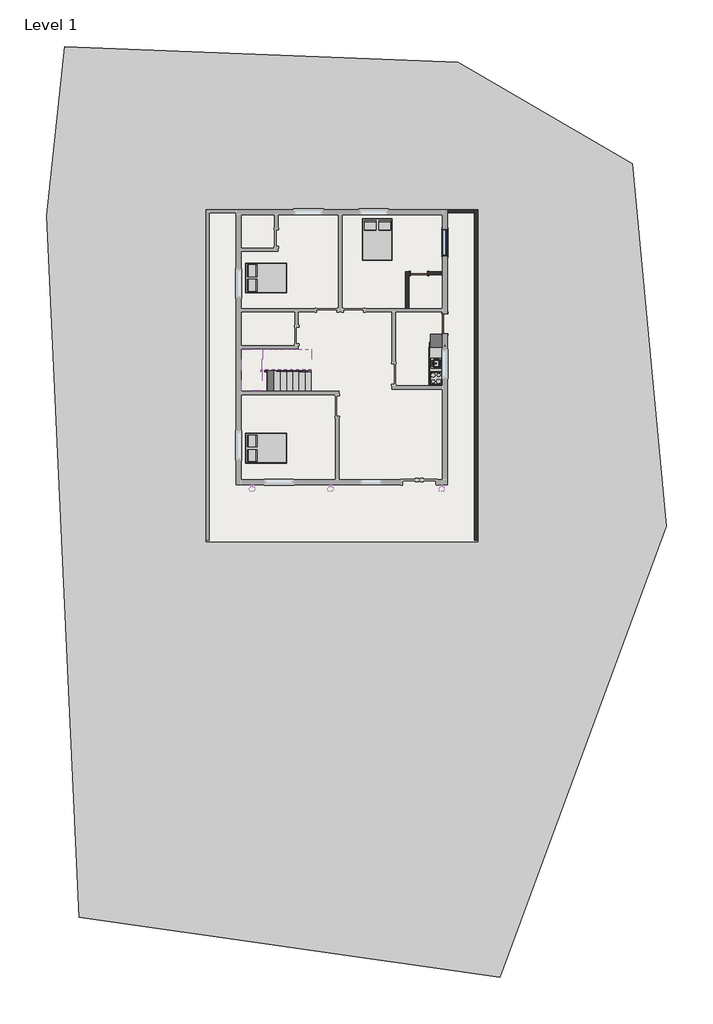
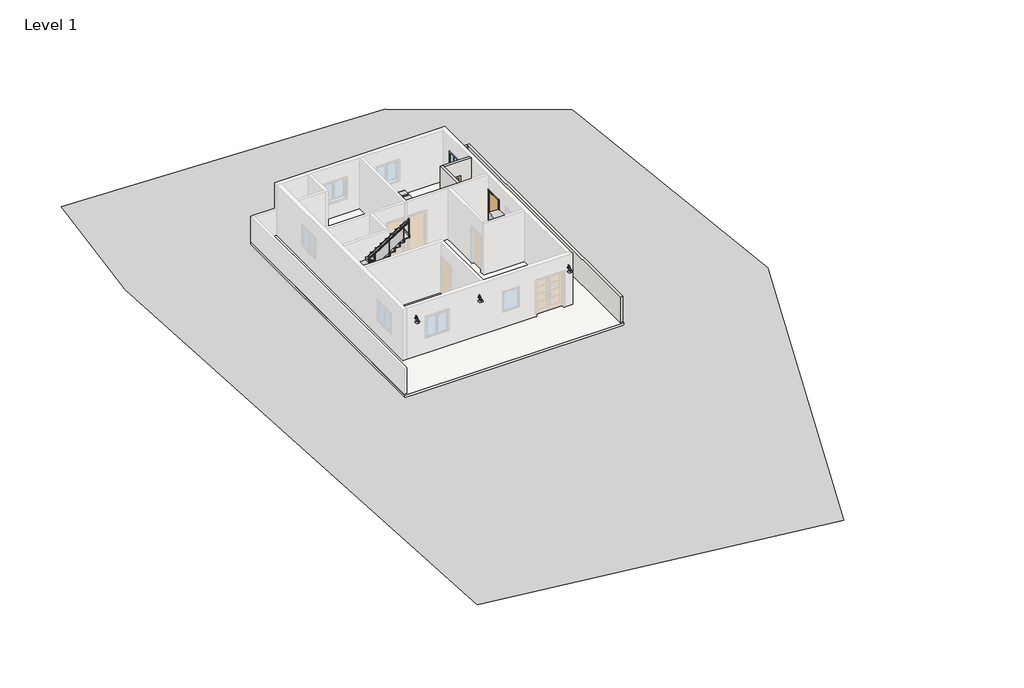
# One storey, part 2 of 2: 5 proxies, 4 furniture elements, 4 walls, 3 light fixtures, 2 doors, 2 members, 2 slabs, 2 stair flights, 3 other elements.
"""IFC4 building model written with IfcOpenShell, lengths in millimetres."""

from ifc_helpers import new_model, si_unit, frame, origin, origin_with_axes, place, context, project, spatial, polyline, outline, extrude, faceted_brep, triangles, transform, mapped, element, save
from components import proxy_a6faaae8, proxy_45b28599, kitchenette_medium_kitchenette_medium_844211aa, proxy_c523a7b7, single_flush_2_5_a9addea7, door_0ca8825f, flow_terminal_871c2e40, furniture_c8abb964, furniture_f14924cf, wall_lamp_bracket_100w_120v_38ba4611, non_monolithic_landing_7588ffe4, stair_flight_6c774f9d, stair_flight_3143a382, window_8af0dca1

model = new_model("IFC4")

# Units and contexts
model_context = context("Model", 3, world=origin())
ifc_project = project(units=[si_unit("LENGTHUNIT", "METRE", prefix="MILLI")], contexts=[model_context])

# Site, building, storey
site = spatial("IfcSite", under=ifc_project)
building = spatial("IfcBuilding", under=site)
storey = spatial("IfcBuildingStorey", under=building, Name="Level 1", Elevation=0.0)

# Proxies
placement = place(None, origin())
element("IfcBuildingElementProxy", 1, Name="Building Element Proxy", at=placement, inside=storey, context=model_context, shape_type="Tessellation", body=[
    triangles([(-15499.5818298, 15063.152655, -152.4), (2359.9797867, 14353.5017853, -152.4), (10284.4210876, 9740.7676437, -152.4), (11821.9993286, -6699.4910706, -152.4), (4274.6428596, -27186.3498779, -152.4), (-14834.2491852, -24452.2749023, -152.4), (-16327.5080383, 7375.2626129, -152.4)], [[1, 7, 2], [4, 7, 6], [4, 2, 7], [3, 2, 4], [4, 6, 5]], closed=False),
])
proxy_shape = proxy_a6faaae8(model_context)
element("IfcBuildingElementProxy", 2, Name="Cook Top-4 Unit2 : 22\" x 20\"", ObjectType="Cook Top-4 Unit2 : 22\" x 20\"", at=placement, inside=storey, context=model_context, shape_type="MappedRepresentation", body=[
    mapped(proxy_shape, transform((1354.3352982, 8.7325188, 0.0), x_axis=(0.0, 1.0000000000000002, 0.0), y_axis=(-1.0000000000000002, 0.0, 0.0), z_axis=(0.0, 0.0, 1.0))),
])
proxy_2_shape = proxy_45b28599(model_context)
element("IfcBuildingElementProxy", 3, Name="Dishwasher : 24\" x 24\" x 34\"", ObjectType="Dishwasher : 24\" x 24\" x 34\"", at=placement, inside=storey, context=model_context, shape_type="MappedRepresentation", body=[
    mapped(proxy_2_shape, transform((1646.184863, 959.9150503, 0.0), x_axis=(0.0, 1.0000000000000002, 0.0), y_axis=(-1.0000000000000002, 0.0, 0.0), z_axis=(0.0, 0.0, 1.0))),
])
kitchenette_medium_kitchenette_medium_shape = kitchenette_medium_kitchenette_medium_844211aa(model_context)
element("IfcBuildingElementProxy", 4, Name="Kitchenette - Medium : Kitchenette - Medium", ObjectType="Kitchenette - Medium : Kitchenette - Medium", at=placement, inside=storey, context=model_context, shape_type="MappedRepresentation", body=[
    mapped(kitchenette_medium_kitchenette_medium_shape, transform((1049.5352982, 332.8948139, 0.0), x_axis=(0.0, 1.0000000000000002, 0.0), y_axis=(-1.0000000000000002, 0.0, 0.0), z_axis=(0.0, 0.0, 1.0))),
])
proxy_3_shape = proxy_c523a7b7(model_context)
element("IfcBuildingElementProxy", 5, Name="Refrigerator : 24\" x 25\" LH", ObjectType="Refrigerator : 24\" x 25\" LH", at=placement, inside=storey, context=model_context, shape_type="MappedRepresentation", body=[
    mapped(proxy_3_shape, transform((1399.9842697, 1716.8825188, 0.0), x_axis=(0.0, 1.0000000000000002, 0.0), y_axis=(-1.0000000000000002, 0.0, 0.0), z_axis=(0.0, 0.0, 1.0))),
])

# Doors
single_flush_2_5_shape = single_flush_2_5_a9addea7(model_context)
element("IfcDoor", 6, ObjectType="Single-Flush : 2.5'", at=placement, inside=storey, context=model_context, shape_type="MappedRepresentation", body=[
    mapped(single_flush_2_5_shape, transform((592.3352982, 4771.2325188, 0.0), x_axis=(-1.0, 0.0, 0.0), y_axis=(0.0, -1.0, 0.0), z_axis=(0.0, 0.0, 1.0))),
])
door_shape = door_0ca8825f(model_context)
element("IfcDoor", 7, ObjectType="Single-Flush : 36\" x 84\"", at=placement, inside=storey, context=model_context, shape_type="MappedRepresentation", body=[
    mapped(door_shape, transform((1773.4352982, 2485.2325188, 0.0), x_axis=(0.0, 1.0, 0.0), y_axis=(-1.0, 0.0, 0.0), z_axis=(0.0, 0.0, 1.0))),
])

# Flow terminal
flow_terminal_shape = flow_terminal_871c2e40(model_context)
element("IfcFlowTerminal", 8, ObjectType="Sink Kitchen-Island : 18\" x 18\"", at=placement, inside=storey, context=model_context, shape_type="MappedRepresentation", body=[
    mapped(flow_terminal_shape, transform((1356.6806993, 666.1432782, -14.4), x_axis=(0.0, 1.0000000000000002, 0.0), y_axis=(-1.0000000000000002, 0.0, 0.0), z_axis=(0.0, 0.0, 1.0))),
])

# Furniture
furniture_shape = furniture_c8abb964(model_context)
element("IfcFurniture", 9, ObjectType="Bed-Box : Double 53\" x 74\"", at=placement, inside=storey, context=model_context, shape_type="MappedRepresentation", body=[
    mapped(furniture_shape, transform((-6588.99421, 4216.1800598, 0.0), x_axis=(0.0, 1.0, 0.0), y_axis=(-1.0, 0.0, 0.0), z_axis=(0.0, 0.0, 1.0))),
])
element("IfcFurniture", 10, ObjectType="Bed-Box : Double 53\" x 74\"", at=placement, inside=storey, context=model_context, shape_type="MappedRepresentation", body=[
    mapped(furniture_shape, transform((-1639.1171608, 6542.362027, 0.0), x_axis=(1.0000000000000004, 0.0, 0.0), y_axis=(0.0, 1.0000000000000004, 0.0), z_axis=(0.0, 0.0, 1.0))),
])
element("IfcFurniture", 11, ObjectType="Bed-Box : Double 53\" x 74\"", at=placement, inside=storey, context=model_context, shape_type="MappedRepresentation", body=[
    mapped(furniture_shape, transform((-6588.99421, -3504.8975153, 0.0), x_axis=(0.0, 1.0, 0.0), y_axis=(-1.0, 0.0, 0.0), z_axis=(0.0, 0.0, 1.0))),
])
furniture_2_shape = furniture_f14924cf(model_context)
element("IfcFurniture", 12, ObjectType="Counter Top w Sink Hole : 24\" Depth", at=placement, inside=storey, context=model_context, shape_type="MappedRepresentation", body=[
    mapped(furniture_2_shape, transform((1049.5352982, 866.2948139, -14.4), x_axis=(0.0, 1.0000000000000002, 0.0), y_axis=(-1.0000000000000002, 0.0, 0.0), z_axis=(0.0, 0.0, 1.0))),
])

# Light fixtures
wall_lamp_bracket_100w_120v_shape = wall_lamp_bracket_100w_120v_38ba4611(model_context)
element("IfcLightFixture", 13, ObjectType="Wall Lamp - Bracket : 100W - 120V", at=placement, inside=storey, context=model_context, shape_type="MappedRepresentation", body=[
    mapped(wall_lamp_bracket_100w_120v_shape, transform((-3461.1148241, -4715.6674812, 0.0), x_axis=(-1.0, 0.0, 0.0), y_axis=(0.0, -1.0, 0.0), z_axis=(0.0, 0.0, 1.0))),
])
element("IfcLightFixture", 14, ObjectType="Wall Lamp - Bracket : 100W - 120V", at=placement, inside=storey, context=model_context, shape_type="MappedRepresentation", body=[
    mapped(wall_lamp_bracket_100w_120v_shape, transform((-7025.9203645, -4715.6674812, 0.0), x_axis=(-1.0, 0.0, 0.0), y_axis=(0.0, -1.0, 0.0), z_axis=(0.0, 0.0, 1.0))),
])
element("IfcLightFixture", 15, ObjectType="Wall Lamp - Bracket : 100W - 120V", at=placement, inside=storey, context=model_context, shape_type="MappedRepresentation", body=[
    mapped(wall_lamp_bracket_100w_120v_shape, transform((1584.6796355, -4715.6674812, 0.0), x_axis=(-1.0, 0.0, 0.0), y_axis=(0.0, -1.0, 0.0), z_axis=(0.0, 0.0, 1.0))),
])

# Members
element("IfcMember", 16, ObjectType="Stringer - 2\" Width", at=placement, inside=storey, context=model_context, shape_type="Brep", body=[
    faceted_brep([(-4345.5091614, 301.3549437, 0.0), (-4543.6146908, 301.3549437, 0.0), (-4543.6146908, 352.1549437, 0.0), (-4345.5091614, 352.1549437, 0.0), (-6548.9591614, 301.3549437, 1371.6), (-6548.9591614, 301.3549437, 1276.1282995), (-4345.5091614, 301.3549437, 127.0), (-4624.9091614, 301.3549437, 127.0), (-4624.9091614, 301.3549437, 304.8), (-4904.3091614, 301.3549437, 304.8), (-4904.3091614, 301.3549437, 482.6), (-5183.7091614, 301.3549437, 482.6), (-5183.7091614, 301.3549437, 660.4), (-5463.1091614, 301.3549437, 660.4), (-5463.1091614, 301.3549437, 838.2), (-5742.5091614, 301.3549437, 838.2), (-5742.5091614, 301.3549437, 1016.0), (-6021.9091614, 301.3549437, 1016.0), (-6021.9091614, 301.3549437, 1193.8), (-6301.3091614, 301.3549437, 1193.8), (-6301.3091614, 301.3549437, 1371.6), (-6548.9591614, 352.1549437, 1276.1282995), (-6548.9591614, 352.1549437, 1371.6), (-6301.3091614, 352.1549437, 1118.532845), (-6021.9091614, 352.1549437, 940.732845), (-5742.5091614, 352.1549437, 762.932845), (-5463.1091614, 352.1549437, 585.132845), (-5183.7091614, 352.1549437, 407.332845), (-4904.3091614, 352.1549437, 229.532845), (-4624.9091614, 352.1549437, 51.732845), (-4345.5091614, 352.1549437, 127.0), (-4624.9091614, 352.1549437, 127.0), (-4624.9091614, 352.1549437, 304.8), (-4904.3091614, 352.1549437, 304.8), (-4904.3091614, 352.1549437, 482.6), (-5183.7091614, 352.1549437, 482.6), (-5183.7091614, 352.1549437, 660.4), (-5463.1091614, 352.1549437, 660.4), (-5463.1091614, 352.1549437, 838.2), (-5742.5091614, 352.1549437, 838.2), (-5742.5091614, 352.1549437, 1016.0), (-6021.9091614, 352.1549437, 1016.0), (-6021.9091614, 352.1549437, 1193.8), (-6301.3091614, 352.1549437, 1193.8), (-6301.3091614, 352.1549437, 1371.6)], [[[0, 1, 2, 3]], [[4, 5, 1, 0, 6, 7, 8, 9, 10, 11, 12, 13, 14, 15, 16, 17, 18, 19, 20]], [[21, 5, 4, 22]], [[5, 21, 23, 24, 25, 26, 27, 28, 29, 2, 1]], [[30, 6, 0, 3]], [[6, 30, 31, 7]], [[7, 31, 32, 8]], [[8, 32, 33, 9]], [[9, 33, 34, 10]], [[10, 34, 35, 11]], [[11, 35, 36, 12]], [[12, 36, 37, 13]], [[13, 37, 38, 14]], [[14, 38, 39, 15]], [[15, 39, 40, 16]], [[16, 40, 41, 17]], [[17, 41, 42, 18]], [[18, 42, 43, 19]], [[19, 43, 44, 20]], [[20, 44, 22, 4]], [[21, 22, 44, 43, 42, 41, 40, 39, 38, 37, 36, 35, 34, 33, 32, 31, 30, 3, 2, 29, 28, 27, 26, 25, 24, 23]]]),
])
element("IfcMember", 17, ObjectType="Stringer - 2\" Width", at=placement, inside=storey, context=model_context, shape_type="SweptSolid", body=[
    extrude(outline(polyline([(-6599.7591614, 402.4325188), (-6548.9591614, 402.4325188), (-6548.9591614, 352.1549437), (-6580.7091614, 352.1549437), (-6580.7091614, 301.3549437), (-6599.7591614, 301.3549437), (-6599.7591614, 402.4325188)])), frame((0.0, 0.0, 1371.6), z_axis=(0.0, 0.0, 1.0), x_axis=(1.0, 0.0, 0.0)), (0.0, 0.0, 1.0), 177.8),
])

# Railing
element("IfcRailing", 18, ObjectType="Glass Panel - Bottom Fill", at=placement, inside=storey, context=model_context, shape_type="SolidModel", body=[
    faceted_brep([(-4313.7591614, 301.3549437, 1092.2), (-4313.7591614, 301.3549437, 1031.986276), (-4313.7591614, 352.1549437, 1031.986276), (-4313.7591614, 352.1549437, 1092.2), (-6548.9591614, 301.3549437, 2514.6), (-6548.9591614, 352.1549437, 2514.6), (-6548.9591614, 352.1549437, 2454.386276), (-6548.9591614, 301.3549437, 2454.386276)], [[[0, 1, 2, 3]], [[4, 5, 6, 7]], [[1, 0, 4, 7]], [[2, 1, 7, 6]], [[3, 2, 6, 5]], [[0, 3, 5, 4]]]),
    faceted_brep([(-6599.7591614, 301.3549437, 2514.6), (-6599.7591614, 301.3549437, 2463.8), (-6548.9591614, 301.3549437, 2463.8), (-6548.9591614, 301.3549437, 2514.6), (-6599.7591614, 402.4325188, 2514.6), (-6548.9591614, 402.4325188, 2514.6), (-6548.9591614, 453.2325188, 2463.8), (-6599.7591614, 453.2325188, 2463.8)], [[[0, 1, 2, 3]], [[4, 5, 6, 7]], [[1, 0, 4, 7]], [[2, 1, 7, 6]], [[3, 2, 6, 5]], [[0, 3, 5, 4]]]),
    faceted_brep([(-6599.7591614, 402.4325188, 2514.6), (-6599.7591614, 453.2325188, 2463.8), (-6548.9591614, 453.2325188, 2463.8), (-6548.9591614, 402.4325188, 2514.6), (-6599.7591614, 402.4325188, 2660.0727273), (-6548.9591614, 402.4325188, 2632.186276), (-6548.9591614, 453.2325188, 2632.186276), (-6599.7591614, 453.2325188, 2660.0727273)], [[[0, 1, 2, 3]], [[4, 5, 6, 7]], [[1, 0, 4, 7]], [[2, 1, 7, 6]], [[3, 2, 6, 5]], [[0, 3, 5, 4]]]),
    faceted_brep([(-6599.7591614, 453.2325188, 2660.0727273), (-6548.9591614, 453.2325188, 2632.186276), (-6548.9591614, 402.4325188, 2632.186276), (-6599.7591614, 402.4325188, 2660.0727273), (-4313.7591614, 453.2325188, 4114.8), (-4313.7591614, 402.4325188, 4114.8), (-4313.7591614, 402.4325188, 4054.586276), (-4313.7591614, 453.2325188, 4054.586276)], [[[0, 1, 2, 3]], [[4, 5, 6, 7]], [[1, 0, 4, 7]], [[2, 1, 7, 6]], [[3, 2, 6, 5]], [[0, 3, 5, 4]]]),
    faceted_brep([(-4313.7591614, 339.4549437, 1005.653431), (-4313.7591614, 314.0549437, 1005.653431), (-4313.7591614, 314.0549437, 975.546569), (-4313.7591614, 339.4549437, 975.546569), (-6545.2609127, 339.4549437, 2425.7), (-6545.2609127, 314.0549437, 2425.7), (-6552.6574102, 314.0549437, 2400.3), (-6552.6574102, 339.4549437, 2400.3), (-6561.6591614, 339.4549437, 2425.7), (-6587.0591614, 314.0549437, 2425.7), (-6587.0591614, 314.0549437, 2400.3), (-6561.6591614, 339.4549437, 2400.3), (-6561.6591614, 415.1325188, 2425.7), (-6561.6591614, 415.1325188, 2400.3), (-6587.0591614, 415.1325188, 2400.3), (-6587.0591614, 415.1325188, 2425.7)], [[[0, 1, 2, 3]], [[1, 0, 4, 5]], [[2, 1, 5, 6]], [[3, 2, 6, 7]], [[0, 3, 7, 4]], [[5, 4, 8, 9]], [[6, 5, 9, 10]], [[7, 6, 10, 11]], [[4, 7, 11, 8]], [[12, 13, 14, 15]], [[9, 8, 12, 15]], [[10, 9, 15, 14]], [[11, 10, 14, 13]], [[8, 11, 13, 12]]]),
    faceted_brep([(-6587.0591614, 415.1325188, 2581.6079765), (-6587.0591614, 440.5325188, 2581.6079765), (-6587.0591614, 440.5325188, 2551.5011144), (-6587.0591614, 415.1325188, 2551.5011144), (-4313.7591614, 415.1325188, 4028.253431), (-4313.7591614, 415.1325188, 3998.146569), (-4313.7591614, 440.5325188, 3998.146569), (-4313.7591614, 440.5325188, 4028.253431)], [[[0, 1, 2, 3]], [[4, 5, 6, 7]], [[1, 0, 4, 7]], [[2, 1, 7, 6]], [[3, 2, 6, 5]], [[0, 3, 5, 4]]]),
    faceted_brep([(-4313.7591614, 339.4549437, 904.053431), (-4313.7591614, 314.0549437, 904.053431), (-4313.7591614, 314.0549437, 873.946569), (-4313.7591614, 339.4549437, 873.946569), (-6545.2609127, 339.4549437, 2324.1), (-6545.2609127, 314.0549437, 2324.1), (-6552.6574102, 314.0549437, 2298.7), (-6552.6574102, 339.4549437, 2298.7), (-6561.6591614, 339.4549437, 2324.1), (-6587.0591614, 314.0549437, 2324.1), (-6587.0591614, 314.0549437, 2298.7), (-6561.6591614, 339.4549437, 2298.7), (-6561.6591614, 415.1325188, 2324.1), (-6561.6591614, 415.1325188, 2298.7), (-6587.0591614, 415.1325188, 2298.7), (-6587.0591614, 415.1325188, 2324.1)], [[[0, 1, 2, 3]], [[1, 0, 4, 5]], [[2, 1, 5, 6]], [[3, 2, 6, 7]], [[0, 3, 7, 4]], [[5, 4, 8, 9]], [[6, 5, 9, 10]], [[7, 6, 10, 11]], [[4, 7, 11, 8]], [[12, 13, 14, 15]], [[9, 8, 12, 15]], [[10, 9, 15, 14]], [[11, 10, 14, 13]], [[8, 11, 13, 12]]]),
    faceted_brep([(-6587.0591614, 415.1325188, 2480.0079765), (-6587.0591614, 440.5325188, 2480.0079765), (-6587.0591614, 440.5325188, 2449.9011144), (-6587.0591614, 415.1325188, 2449.9011144), (-4313.7591614, 415.1325188, 3926.653431), (-4313.7591614, 415.1325188, 3896.546569), (-4313.7591614, 440.5325188, 3896.546569), (-4313.7591614, 440.5325188, 3926.653431)], [[[0, 1, 2, 3]], [[4, 5, 6, 7]], [[1, 0, 4, 7]], [[2, 1, 7, 6]], [[3, 2, 6, 5]], [[0, 3, 5, 4]]]),
    extrude(outline(polyline([(3856.5817305, -4624.9091614), (3848.4999123, -4637.6091614), (2844.8, -4637.6091614), (2844.8, -4624.9091614), (3856.5817305, -4624.9091614)])), frame((0.0, 402.4325188, 0.0), z_axis=(0.0, 1.0, 0.0), x_axis=(0.0, 0.0, 1.0)), (0.0, 0.0, 1.0), 50.8),
    extrude(outline(polyline([(2509.9818182, -5444.0591614), (3027.2181818, -4631.2591614), (3694.5011144, -4631.2591614), (3177.2647508, -5444.0591614), (2509.9818182, -5444.0591614)])), frame((0.0, 428.0176758, 0.0), z_axis=(0.0, 1.0, 0.0), x_axis=(0.0, 0.0, 1.0)), (0.0, 0.0, 1.0), 6.35),
    extrude(outline(polyline([(3339.3453669, -5437.7091614), (3331.2635487, -5450.4091614), (2311.4, -5450.4091614), (2311.4, -5437.7091614), (3339.3453669, -5437.7091614)])), frame((0.0, 402.4325188, 0.0), z_axis=(0.0, 1.0, 0.0), x_axis=(0.0, 0.0, 1.0)), (0.0, 0.0, 1.0), 50.8),
    extrude(outline(polyline([(1976.5818182, -6256.8591614), (2493.8181818, -5444.0591614), (3177.2647508, -5444.0591614), (2660.0283872, -6256.8591614), (1976.5818182, -6256.8591614)])), frame((0.0, 428.0176758, 0.0), z_axis=(0.0, 1.0, 0.0), x_axis=(0.0, 0.0, 1.0)), (0.0, 0.0, 1.0), 6.35),
    extrude(outline(polyline([(2822.1090032, -6250.5091614), (2814.0271851, -6263.2091614), (1955.8, -6263.2091614), (1955.8, -6250.5091614), (2822.1090032, -6250.5091614)])), frame((0.0, 402.4325188, 0.0), z_axis=(0.0, 1.0, 0.0), x_axis=(0.0, 0.0, 1.0)), (0.0, 0.0, 1.0), 50.8),
    extrude(outline(polyline([(2256.3817305, -6237.8091614), (2264.4635487, -6250.5091614), (1244.6, -6250.5091614), (1244.6, -6237.8091614), (2256.3817305, -6237.8091614)])), frame((0.0, 301.3549437, 0.0), z_axis=(0.0, 1.0, 0.0), x_axis=(0.0, 0.0, 1.0)), (0.0, 0.0, 1.0), 50.8),
    extrude(outline(polyline([(909.7818182, -5431.3591614), (1585.146569, -5431.3591614), (2102.3829326, -6244.1591614), (1427.0181818, -6244.1591614), (909.7818182, -5431.3591614)])), frame((0.0, 320.2197867, 0.0), z_axis=(0.0, 1.0, 0.0), x_axis=(0.0, 0.0, 1.0)), (0.0, 0.0, 1.0), 6.35),
    extrude(outline(polyline([(1739.1453669, -5425.0091614), (1747.2271851, -5437.7091614), (889.0, -5437.7091614), (889.0, -5425.0091614), (1739.1453669, -5425.0091614)])), frame((0.0, 301.3549437, 0.0), z_axis=(0.0, 1.0, 0.0), x_axis=(0.0, 0.0, 1.0)), (0.0, 0.0, 1.0), 50.8),
    extrude(outline(polyline([(376.3818182, -4618.5591614), (1067.9102054, -4618.5591614), (1585.146569, -5431.3591614), (893.6181818, -5431.3591614), (376.3818182, -4618.5591614)])), frame((0.0, 320.2197867, 0.0), z_axis=(0.0, 1.0, 0.0), x_axis=(0.0, 0.0, 1.0)), (0.0, 0.0, 1.0), 6.35),
    extrude(outline(polyline([(1221.9090032, -4612.2091614), (1229.9908214, -4624.9091614), (355.6, -4624.9091614), (355.6, -4612.2091614), (1221.9090032, -4612.2091614)])), frame((0.0, 301.3549437, 0.0), z_axis=(0.0, 1.0, 0.0), x_axis=(0.0, 0.0, 1.0)), (0.0, 0.0, 1.0), 50.8),
    extrude(outline(polyline([(-6583.8841614, 418.3075188), (-6583.8841614, 437.3575188), (-6564.8341614, 437.3575188), (-6564.8341614, 418.3075188), (-6583.8841614, 418.3075188)])), frame((0.0, 0.0, 1600.2), z_axis=(0.0, 0.0, 1.0), x_axis=(1.0, 0.0, 0.0)), (0.0, 0.0, 1.0), 863.6),
    extrude(outline(polyline([(2464.4885487, -6564.8341614), (2476.611276, -6583.8841614), (1600.2, -6583.8841614), (1600.2, -6564.8341614), (2464.4885487, -6564.8341614)])), frame((0.0, 317.2299437, 0.0), z_axis=(0.0, 1.0, 0.0), x_axis=(0.0, 0.0, 1.0)), (0.0, 0.0, 1.0), 19.05),
    extrude(outline(polyline([(2448.3249123, -6539.4341614), (2460.4476396, -6558.4841614), (1600.2, -6558.4841614), (1600.2, -6539.4341614), (2448.3249123, -6539.4341614)])), frame((0.0, 317.2299437, 0.0), z_axis=(0.0, 1.0, 0.0), x_axis=(0.0, 0.0, 1.0)), (0.0, 0.0, 1.0), 19.05),
    extrude(outline(polyline([(4058.6271851, -4307.4091614), (4046.5044578, -4326.4591614), (3022.6, -4326.4591614), (3022.6, -4307.4091614), (4058.6271851, -4307.4091614)])), frame((0.0, 418.3075188, 0.0), z_axis=(0.0, 1.0, 0.0), x_axis=(0.0, 0.0, 1.0)), (0.0, 0.0, 1.0), 19.05),
    extrude(outline(polyline([(1027.9453669, -4307.4091614), (1040.0680941, -4326.4591614), (177.8, -4326.4591614), (177.8, -4307.4091614), (1027.9453669, -4307.4091614)])), frame((0.0, 317.2299437, 0.0), z_axis=(0.0, 1.0, 0.0), x_axis=(0.0, 0.0, 1.0)), (0.0, 0.0, 1.0), 19.05),
])

# Slabs
element("IfcSlab", 19, ObjectType="6\"", at=placement, inside=storey, context=model_context, shape_type="SweptSolid", body=[
    extrude(outline(polyline([(3259.3352982, 7666.8325188), (3259.3352982, -7420.7674812), (-9085.0647018, -7420.7674812), (-9085.0647018, 7666.8325188), (3259.3352982, 7666.8325188)])), frame((0.0, 0.0, -152.4), z_axis=(0.0, 0.0, 1.0), x_axis=(1.0, 0.0, 0.0)), (0.0, 0.0, 1.0), 152.4),
])
non_monolithic_landing_shape = non_monolithic_landing_7588ffe4(model_context)
element("IfcSlab", 20, ObjectType="Non-Monolithic Landing", at=placement, inside=storey, context=model_context, shape_type="MappedRepresentation", body=[
    mapped(non_monolithic_landing_shape, transform((0.0, 0.0, 0.0), x_axis=(1.0, 0.0, 0.0), y_axis=(0.0, 1.0, 0.0), z_axis=(0.0, 0.0, 1.0))),
])

# Stair flights
stair_flight_shape = stair_flight_6c774f9d(model_context)
element("IfcStairFlight", 21, ObjectType="2\" Tread 1\" Nosing 1/4\" Riser", at=placement, inside=storey, context=model_context, shape_type="MappedRepresentation", body=[
    mapped(stair_flight_shape, transform((0.0, 0.0, 0.0), x_axis=(1.0, 0.0, 0.0), y_axis=(0.0, 1.0, 0.0), z_axis=(0.0, 0.0, 1.0))),
])
stair_flight_2_shape = stair_flight_3143a382(model_context)
element("IfcStairFlight", 22, ObjectType="2\" Tread 1\" Nosing 1/4\" Riser", at=placement, inside=storey, context=model_context, shape_type="MappedRepresentation", body=[
    mapped(stair_flight_2_shape, transform((0.0, 0.0, 0.0), x_axis=(1.0, 0.0, 0.0), y_axis=(0.0, 1.0, 0.0), z_axis=(0.0, 0.0, 1.0))),
])

# Walls
element("IfcWall", 23, ObjectType="6\"", at=placement, inside=storey, context=model_context, shape_type="Brep", body=[
    faceted_brep([(3106.9352982, 7666.8325188, 0.0), (3106.9352982, 7514.4325188, 0.0), (3106.9352982, -7344.5674812, 0.0), (3106.9352982, -7344.5674812, 1524.0), (3106.9352982, 7514.4325188, 1524.0), (3106.9352982, 7666.8325188, 1524.0), (3259.3352982, 7666.8325188, 0.0), (3259.3352982, 7666.8325188, 1524.0), (3259.3352982, -7344.5674812, 1524.0), (3259.3352982, -7344.5674812, 0.0)], [[[0, 1, 2, 3, 4, 5]], [[6, 7, 8, 9]], [[2, 1, 0, 6, 9]], [[3, 2, 9, 8]], [[5, 4, 3, 8, 7]], [[0, 5, 7, 6]]]),
])
element("IfcWall", 24, ObjectType="6\"", at=placement, inside=storey, context=model_context, shape_type="Brep", body=[
    faceted_brep([(135.1352982, 3171.0325188, 0.0), (135.1352982, 4695.0325188, 0.0), (135.1352982, 4847.4325188, 0.0), (135.1352982, 4847.4325188, 3048.0), (135.1352982, 4695.0325188, 3048.0), (135.1352982, 3171.0325188, 3048.0), (-17.2647018, 3171.0325188, 0.0), (-17.2647018, 3171.0325188, 3048.0), (-17.2647018, 4847.4325188, 3048.0), (-17.2647018, 4847.4325188, 0.0)], [[[0, 1, 2, 3, 4, 5]], [[6, 7, 8, 9]], [[2, 1, 0, 6, 9]], [[5, 4, 3, 8, 7]], [[0, 5, 7, 6]], [[3, 2, 9, 8]]]),
])
element("IfcWall", 25, ObjectType="6\"", at=placement, inside=storey, context=model_context, shape_type="SweptSolid", body=[
    extrude(outline(polyline([(0.0, 135.1352982), (0.0, 211.3352982), (2133.6, 211.3352982), (2133.6, 973.3352982), (0.0, 973.3352982), (0.0, 1659.1352982), (3048.0, 1659.1352982), (3048.0, 135.1352982), (0.0, 135.1352982)])), frame((0.0, 4695.0325188, 0.0), z_axis=(0.0, 1.0, 0.0), x_axis=(0.0, 0.0, 1.0)), (0.0, 0.0, 1.0), 152.4),
])
element("IfcWall", 26, ObjectType="6\"", at=placement, inside=storey, context=model_context, shape_type="SweptSolid", body=[
    extrude(outline(polyline([(3106.9352982, 7514.4325188), (1887.7352982, 7514.4325188), (1887.7352982, 7666.8325188), (3106.9352982, 7666.8325188), (3106.9352982, 7514.4325188)])), origin_with_axes(), (0.0, 0.0, 1.0), 1524.0),
])

# Window
window_shape = window_8af0dca1(model_context)
element("IfcWindow", 27, ObjectType="Casement Dbl with Trim : 48\" x 48\"", at=placement, inside=storey, context=model_context, shape_type="MappedRepresentation", body=[
    mapped(window_shape, transform((1754.3852982, 6161.8825188, 152.4), x_axis=(0.0, -1.0, 0.0), y_axis=(1.0, 0.0, 0.0), z_axis=(0.0, 0.0, 1.0))),
])

save(model, "model.ifc")

# Revit data of these elements
# Type "Cook Top-4 Unit2 : 22\" x 20\""
#   Depth = 1' - 8"
#   Width = 1' - 10"
#   Burner Material = Steel, Chrome Plated
#   Cooktop Material = Steel, Polished
#   Default Elevation = 0
#   Assembly Code = ""
# Type "Dishwasher : 24\" x 24\" x 34\""
#   Label = "DW"
#   Assembly Code = "E1090400"
#   Depth = 2' - 0"
#   Height = 2' - 10"
#   Width = 2' - 0"
#   Dishwasher Material = Steel, Paint Finish, Ivory, Glossy
#   Panel Face Material = Plastic, Opaque Black
#   Default Elevation = 0
# Type "Kitchenette - Medium : Kitchenette - Medium"
#   Assembly Code = "E1090400"
#   Counter Length = 5' - 9"
#   Cabinet Width = 4' - 6"
#   Cabinet Height = 2' - 10 1/2"
#   Cabinet Depth = 2' - 0"
#   Toe Depth = 0' - 3"
#   Toe Height = 0' - 3 1/2"
#   Cabinet Material = Cabinets
#   Door/Drawer Material = Cabinets
#   Handle Material = Cabinets - Handles
#   Default Elevation = 0
# Type "Refrigerator : 24\" x 25\" LH"
#   Label = "REF."
#   Assembly Code = "E1090400"
#   Depth = 2' - 0 3/4"
#   Handle = 0' - 1 1/2"
#   Height = 5' - 3 1/2"
#   Rear Clearance = 0' - 2"
#   Top Door Height = 1' - 8"
#   Width = 1' - 11 1/2"
#   Material = Steel, Paint Finish, Ivory, Glossy
#   Default Elevation = 0
# Type "Single-Flush : 2.5'"
#   Type Mark = "8"
#   Construction Type Id = "MDOOR"
#   Assembly Code = "C1020"
#   Analytic Construction = "Metal"
#   Thickness = 0' - 2"
#   Heat Transfer Coefficient (U) = 0.651978 BTU/(h·ft²·°F)
#   Height = 7' - 0"
#   Trim Projection Ext = 0' - 1"
#   Trim Projection Int = 0' - 1"
#   Trim Width = 0' - 3"
#   Width = 2' - 6"
#   Define Thermal Properties by = 1
#   Door Material = Door - Panel
#   Frame Material = Door - Frame
#   Visual Light Transmittance = 0
#   Solar Heat Gain Coefficient = 0
#   Function = (empty or 0)
#   Wall Closure = (empty or 0)
# Type "Single-Flush : 36\" x 84\""
#   Type Mark = "1"
#   Construction Type Id = "MDOOR"
#   Assembly Code = "C1020"
#   Analytic Construction = "Metal"
#   Thickness = 0' - 2"
#   Heat Transfer Coefficient (U) = 0.651978 BTU/(h·ft²·°F)
#   Height = 7' - 0"
#   Trim Projection Ext = 0' - 1"
#   Trim Projection Int = 0' - 1"
#   Trim Width = 0' - 3"
#   Width = 3' - 0"
#   Define Thermal Properties by = 1
#   Door Material = Door - Panel
#   Frame Material = Door - Frame
#   Visual Light Transmittance = 0
#   Solar Heat Gain Coefficient = 0
#   Function = (empty or 0)
#   Wall Closure = (empty or 0)
# Type "Sink Kitchen-Island : 18\" x 18\""
#   Assembly Code = "D2010410"
#   Counter Height = 3' - 0"
#   Depth = 1' - 6"
#   Width = 1' - 6"
#   Faucet Material = Steel, Polished
#   Sink Material = Steel, Polished
#   Default Elevation = 0
# Type "Bed-Box : Double 53\" x 74\""
#   Assembly Code = "E2020200"
#   Length = 6' - 2"
#   Width = 4' - 5"
#   Frame Material = Birch
#   Mattress Material = Linen, White
#   Default Elevation = 0
# Type "Counter Top w Sink Hole : 24\" Depth"
#   Assembly Code = "C1030400"
#   Counter Thickness = 0' - 1 1/2"
#   Depth = 2' - 1"
#   Height = 3' - 0"
#   Length [instance default] = 8' - 0"
#   Sink Location [instance default] = 2' - 0"
#   Sink Location To Wall [instance default] = 0' - 6"
#   Sink Opening Depth [instance default] = 1' - 3"
#   Sink Opening Width [instance default] = 2' - 3"
#   Counter Top Material = none
#   Default Elevation = 0
# Type "Wall Lamp - Bracket : 100W - 120V"
#   Lamp = "A-19"
#   Assembly Code = "D5020220"
#   Wattage = 100 W
#   built-in parameter 1150110 = 1 (stored number, unit not read)
#   built-in parameter 1114217 = 1 (stored number, unit not read)
#   built-in parameter 1150109 = 1 (stored number, unit not read)
#   built-in parameter 1150113 = 1 (stored number, unit not read)
#   built-in parameter 1150115 = 1 (stored number, unit not read)
#   built-in parameter 1150105 = 134.486 (stored number, unit not read)
#   Light Source Symbol Size = 2' - 0"
#   built-in parameter 1150112 = 1 (stored number, unit not read)
#   built-in parameter 1150114 = 1 (stored number, unit not read)
#   built-in parameter 1150107 = 2800 (stored number, unit not read)
#   built-in parameter 1150106 = 1.34486 (stored number, unit not read)
#   built-in parameter 1150104 = 1.57006 (stored number, unit not read)
#   Ballast Voltage = 120 V
#   built-in parameter 1114218 = 1 (stored number, unit not read)
#   built-in parameter 1150133 = 10 (stored number, unit not read)
#   Lumens = 1690 lm
#   Apparent Load = 100 VA
#   built-in parameter 1150134 = 4
#   built-in parameter 1150137 = 1
#   Color Filter = 16777215
#   built-in parameter 1140040 [instance default] = 1
#   Ballast Number of Poles = 1
#   Bulb Material = Glass, White, High Luminance
#   Shade Material = Glass, Frosted
#   Wall Mount Material = Steel, Chrome Plated
#   Dimming Lamp Color Temperature Shift = (empty or 0)
#   Default Elevation = 0
#   Wattage Comments = ""
# Type "Glass Panel - Bottom Fill"
#   Assembly Code = "C2010400"
#   built-in parameter 1008612 = 0.0416667 (stored number, unit not read)
#   built-in parameter 1008611 = 0.0416667 (stored number, unit not read)
#   built-in parameter 1008609 = 0.333333 (stored number, unit not read)
#   built-in parameter 1008604 = 0.166667 (stored number, unit not read)
#   built-in parameter 1008603 = 0.166667 (stored number, unit not read)
#   Railing Height = 3' - 0"
#   built-in parameter 1008630 = 2
#   built-in parameter 1008610 = 2
#   built-in parameter 1008618 = Baluster - Square : 3/4"
# Type "6\""
#   Assembly Code = "B1010"
#   Function = 0
#   Layers, outside or top first: 0' - 6" "floor" (function 1)
# Type "6\""
#   Assembly Code = "B2010"
#   Layers, outside or top first: 0' - 6" "inner wall" (function 1)
# Type "Casement Dbl with Trim : 48\" x 48\""
#   Type Mark = "10"
#   Construction Type Id = "GSP4R"
#   Assembly Code = "B2020100"
#   Analytic Construction = "1/8 in Pilkington single glazing"
#   Visual Light Transmittance = 0.9
#   Solar Heat Gain Coefficient = 0.78
#   Heat Transfer Coefficient (U) = 0.6496 BTU/(h·ft²·°F)
#   Height = 4' - 0"
#   Default Sill Height = 2' - 6"
#   Trim Projection - Ext. = 0' - 0 1/2"
#   Trim Projection - Int. = 0' - 0 3/4"
#   Trim Width - Exterior = 0' - 3 1/2"
#   Trim Width - Interior = 0' - 3 1/2"
#   Width = 4' - 0"
#   Window Inset = 0' - 0 3/4"
#   Define Thermal Properties by = 1
#   Glass Pane Material = Glass
#   Sash Material = Sash
#   Trim Exterior Material = Trim
#   Trim Interior Material = Trim
#   Wall Closure = (empty or 0)
# Element 1 (IfcBuildingElementProxy)
#   Material = grass
#   Phase Created = New Construction
# Element 2 (IfcBuildingElementProxy, "Cook Top-4 Unit2 : 22\" x 20\"")
#   Phase Created = New Construction
#   Materials on its faces: "Steel, Chrome Plated", "Steel, Polished"
# Element 3 (IfcBuildingElementProxy, "Dishwasher : 24\" x 24\" x 34\"")
#   Phase Created = New Construction
#   Materials on its faces: "Steel, Paint Finish, Ivory, Glossy", "Plastic, Opaque Black"
# Element 4 (IfcBuildingElementProxy, "Kitchenette - Medium : Kitchenette - Medium")
#   Phase Created = New Construction
#   Materials on its faces: "Cabinets", "Cabinets - Handles"
# Element 5 (IfcBuildingElementProxy, "Refrigerator : 24\" x 25\" LH")
#   Phase Created = New Construction
#   Materials on its faces: "Steel, Paint Finish, Ivory, Glossy", "Steel, Chrome Plated"
# Element 6 (IfcDoor, "Single-Flush : 2.5'")
#   Phase Created = New Construction
#   Materials on its faces: "Door - Frame", "Door - Panel"
# Element 7 (IfcDoor, "Single-Flush : 36\" x 84\"")
#   Phase Created = New Construction
#   Materials on its faces: "Door - Frame", "Door - Panel"
# Element 8 (IfcFlowTerminal, "Sink Kitchen-Island : 18\" x 18\"")
#   Mark = "7"
#   Phase Created = New Construction
#   Materials on its faces: "Steel, Polished"
# Elements 9, 10, 11 (IfcFurniture, "Bed-Box : Double 53\" x 74\"")
#   Phase Created = New Construction
#   Materials on its faces: "Birch", "Linen, White"
# Element 12 (IfcFurniture, "Counter Top w Sink Hole : 24\" Depth")
#   Sink Opening Depth = 1' - 2"
#   Sink Location To Wall = 0' - 6"
#   Length = 5' - 9"
#   Sink Location = 3' - 4"
#   Sink Opening Width = 1' - 4"
#   Phase Created = New Construction
#   Materials on its faces: "Counter Top"
# Element 13 (IfcLightFixture, "Wall Lamp - Bracket : 100W - 120V")
#   Mark = "1"
#   built-in parameter 1140040 = 1
#   Phase Created = New Construction
#   Materials on its faces: "Steel, Chrome Plated", "Glass, Frosted", "Glass, White, High Luminance"
# Element 14 (IfcLightFixture, "Wall Lamp - Bracket : 100W - 120V")
#   Mark = "2"
#   built-in parameter 1140040 = 1
#   Phase Created = New Construction
#   Materials on its faces: "Steel, Chrome Plated", "Glass, Frosted", "Glass, White, High Luminance"
# Element 15 (IfcLightFixture, "Wall Lamp - Bracket : 100W - 120V")
#   Mark = "3"
#   built-in parameter 1140040 = 1
#   Phase Created = New Construction
#   Materials on its faces: "Steel, Chrome Plated", "Glass, Frosted", "Glass, White, High Luminance"
# Elements 16, 17 (IfcMember, "Stringer - 2\" Width")
#   Phase Created = New Construction
# Element 18 (IfcRailing, "Glass Panel - Bottom Fill")
#   Phase Created = New Construction
#   Materials on its faces: "Glass"
# Element 19 (IfcSlab, "6\"")
#   Height Offset From Level = 0' - 0"
#   Phase Created = New Construction
#   Materials on its faces: "floor"
# Element 20 (IfcSlab, "Non-Monolithic Landing")
#   Phase Created = New Construction
# Elements 21, 22 (IfcStairFlight, "2\" Tread 1\" Nosing 1/4\" Riser")
#   Phase Created = New Construction
# Elements 23, 26 (IfcWall, "6\"")
#   Top Offset = 0' - 0"
#   Base Offset = 0' - 0"
#   Unconnected Height = 5' - 0"
#   wall height = 5' - 0"
#   Phase Created = New Construction
#   Base Constraint = Level 1
#   Materials on its faces: "inner wall"
# Elements 24, 25 (IfcWall, "6\"")
#   Top Offset = 0' - 0"
#   Base Offset = 0' - 0"
#   Unconnected Height = 10' - 0"
#   wall height = 10' - 0"
#   Phase Created = New Construction
#   Base Constraint = Level 1
#   Materials on its faces: "inner wall"
# Element 27 (IfcWindow, "Casement Dbl with Trim : 48\" x 48\"")
#   Mark = "7"
#   Phase Created = New Construction
#   Materials on its faces: "Sash", "Trim", "Glass"
# Materials
#   "Steel, Chrome Plated": class "Metal", colour RGB 17 17 17, transparency 0, Description = "Chromiuim plated steel", Cost = 0
#   "Steel, Polished": class "Metal", colour RGB 57 57 57, transparency 0, Description = "Polished steel", Cost = 0
#   "Steel, Paint Finish, Ivory, Glossy": class "Metal", colour RGB 247 247 239, transparency 0, Description = "Steel, paint finish, ivory, glossy", Cost = 0
#   "Plastic, Opaque Black": class "Plastic", colour RGB 0 0 0, transparency 0.7, Description = "Plastic, generic, opaque black", Cost = 0
#   "Cabinets": colour RGB 249 249 249, transparency 0
#   "Cabinets - Handles": class "Metal", colour RGB 57 57 57, transparency 0
#   "Door - Panel": class "Wood", colour RGB 210 159 95, transparency 0
#   "Door - Frame": colour RGB 118 70 51, transparency 0
#   "Birch": class "Wood", colour RGB 224 178 126, transparency 0, Description = "Betula Alleghaniensis", Cost = 0
#   "Linen, White": class "Textile", colour RGB 247 247 239, transparency 0, Description = "Linen, white", Cost = 0
#   "Glass, White, High Luminance": class "Glass", colour RGB 249 250 249, transparency 0.8, Description = "physical material", Cost = 0
#   "Glass, Frosted": class "Glass", colour RGB 250 244 225, transparency 0.55, Description = "physical material", Cost = 0
#   "floor": class "Generic", colour RGB 128 100 74, transparency 0, Cost = 0
#   "inner wall": class "Generic", colour RGB 230 213 172, transparency 0, Cost = 0
#   "Glass": class "Glass", colour RGB 0 128 192, transparency 0.75, Description = "Soda Lime Glass", Cost = 0
#   "Sash": class "Wood", colour RGB 224 178 126, transparency 0
#   "Trim": class "Wood", colour RGB 224 178 126, transparency 0
#   "grass": class "Generic", colour RGB 127 136 91, transparency 0, Cost = 0
#   "Counter Top": class "Wood", colour RGB 226 177 128, transparency 0
